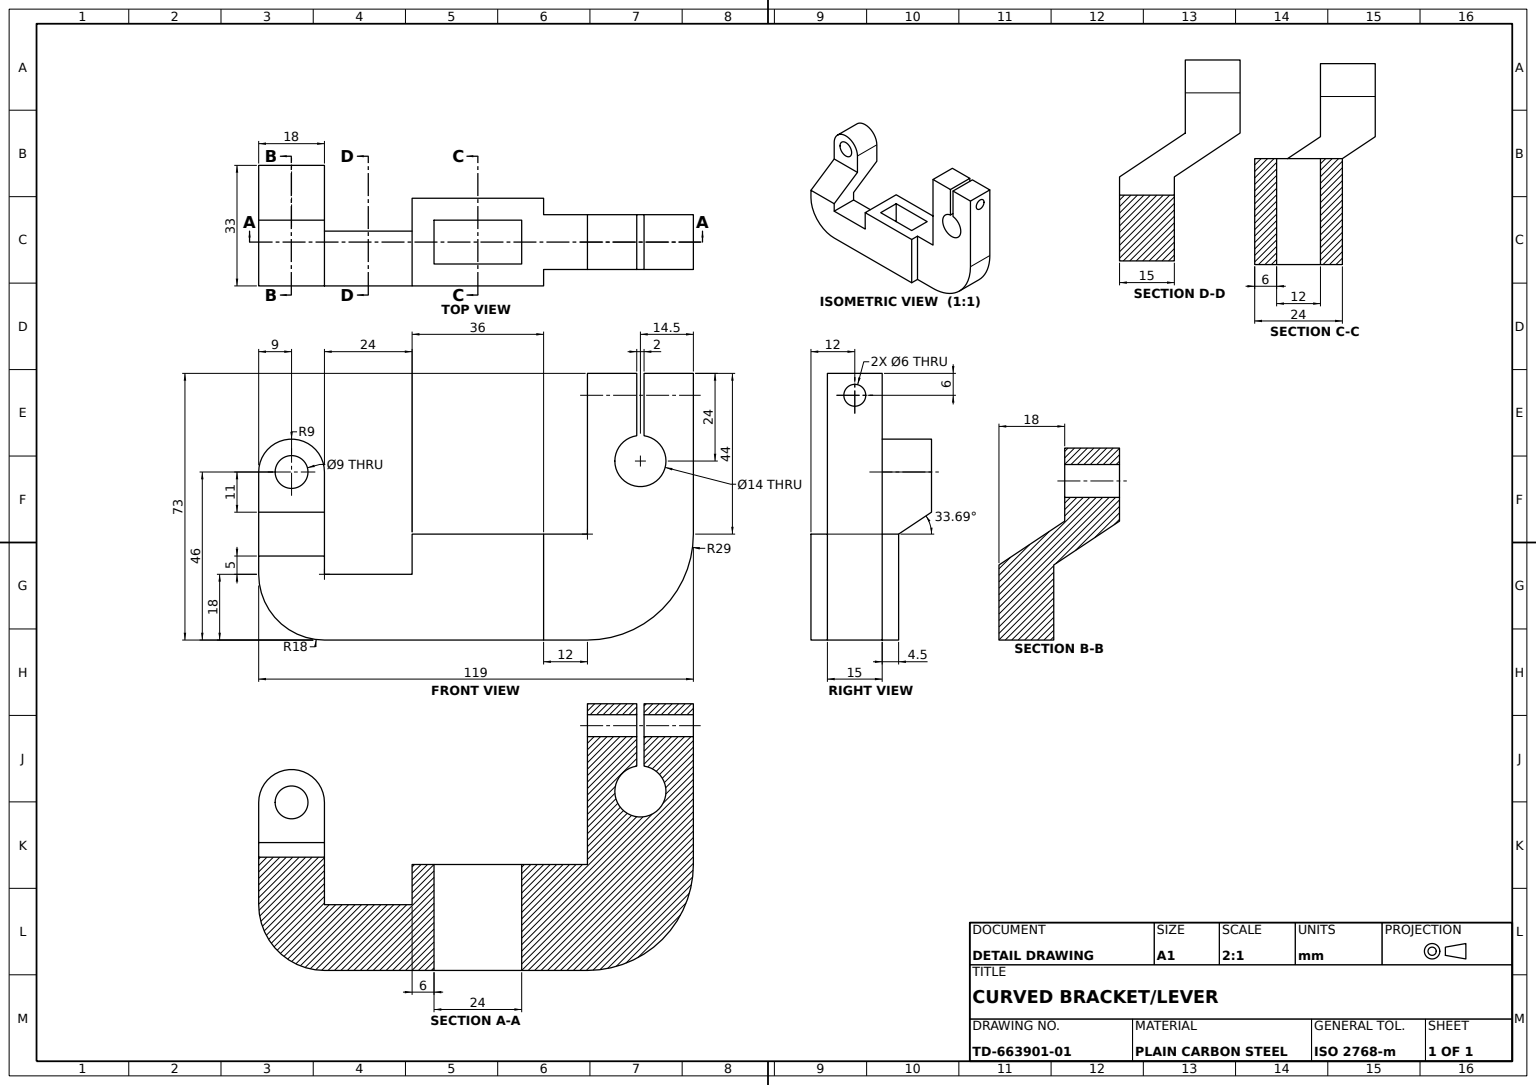
from build123d import *

# Parameters (mm, degrees)
BRACKET_BODY_DEPTH         = 12
BODY_RELIEF_CUT_DEPTH      = 75.57211275
BODY_RELIEF_CUT_DEPTH_BACK = 75.57211275
BODY_RELIEF_SKETCH_W       = 24
BODY_RELIEF_SKETCH_H       = 12
BODY_RELIEF_SKETCH_H_2     = 9
BODY_RELIEF_SKETCH_W_2     = 41
BODY_RELIEF_SKETCH_H_3     = 4.5
RECTANGULAR_WINDOW_DEPTH   = 86.343423883
CLAMP_HOLE_SKETCH_R        = 3
CLAMP_HOLE_6_DEPTH         = 94.542770966
ARM_BOSS_DEPTH             = 15
PIVOT_LUG_DEPTH            = 18
LUG_FILL_BOSS_DEPTH        = 15
PIVOT_BORE_SKETCH_R        = 4.5
PIVOT_BORE_9_DEPTH         = 24


with BuildPart() as part:
    # Bracket Profile Sketch → Bracket Body (new, symmetric)
    with BuildSketch(Plane.XY):
        with BuildLine():
            Line((30, 14.5), (30, 58.5))
            Line((30, 58.5), (59, 58.5))
            Line((59, 58.5), (59, 14.5))
            ThreePointArc((59, 14.5), (50.506096654, -6.006096654), (30, -14.5))
            Line((30, -14.5), (18, -14.5))
            Line((18, -14.5), (-18, -14.5))
            Line((-18, -14.5), (-42, -14.5))
            Line((-42, -14.5), (-42, 3.5))
            Line((-42, 3.5), (-18, 3.5))
            Line((-18, 3.5), (-18, 14.5))
            Line((-18, 14.5), (18, 14.5))
            Line((18, 14.5), (30, 14.5))
        make_face()
    extrude(amount=BRACKET_BODY_DEPTH, both=True)

    # Body Relief Sketch → Body Relief Cut (cut, two sides: drawn at the far end of the back side and taken through both)
    with BuildSketch(Plane(origin=(0, 14.5, 0), x_dir=(1, 0, 0), z_dir=(0, 1, 0)).offset(-BODY_RELIEF_CUT_DEPTH_BACK)):
        Rectangle(BODY_RELIEF_SKETCH_W, BODY_RELIEF_SKETCH_H)
        with Locations((-30, 7.5)):
            Rectangle(BODY_RELIEF_SKETCH_W, BODY_RELIEF_SKETCH_H_2)
        with Locations((38.5, -9.75)):
            Rectangle(BODY_RELIEF_SKETCH_W_2, BODY_RELIEF_SKETCH_H_3)
        with Locations((38.5, 9.75)):
            Rectangle(BODY_RELIEF_SKETCH_W_2, BODY_RELIEF_SKETCH_H_3)
    extrude(amount=BODY_RELIEF_CUT_DEPTH + BODY_RELIEF_CUT_DEPTH_BACK, mode=Mode.SUBTRACT)

    # Window Sketch → Rectangular Window (cut, through all)
    with BuildSketch(Plane.XY.offset(7.5)):
        with BuildLine():
            Line((43.5, 41.42820323), (43.5, 58.5))
            Line((43.5, 58.5), (45.5, 58.5))
            Line((45.5, 58.5), (45.5, 41.42820323))
            ThreePointArc((45.5, 41.42820323), (44.5, 27.5), (43.5, 41.42820323))
        make_face()
    extrude(amount=-RECTANGULAR_WINDOW_DEPTH, mode=Mode.SUBTRACT)

    # Clamp Hole Sketch → Clamp Hole Ø6 (cut, through all)
    with BuildSketch(Plane.ZY.offset(-30)):
        with Locations((0, 52.5)):
            Circle(CLAMP_HOLE_SKETCH_R)
    extrude(amount=-CLAMP_HOLE_6_DEPTH, mode=Mode.SUBTRACT)

    # Arm Sketch → Arm Boss (add)
    with BuildSketch(Plane.XY.offset(12)):
        with BuildLine():
            Line((-60, 3.5), (-60, 8.5))
            Line((-60, 8.5), (-42, 8.5))
            Line((-42, 8.5), (-42, 3.5))
            Line((-42, 3.5), (-42, -14.5))
            ThreePointArc((-42, -14.5), (-54.727922061, -9.227922061), (-60, 3.5))
        make_face()
    extrude(amount=-ARM_BOSS_DEPTH)

    # Pivot Lug Sketch → Pivot Lug (add)
    with BuildSketch(Plane.ZY.offset(60)):
        Polygon((-3, 8.5), (-21, 20.5), (-21, 31.5), (-6, 31.5), (-6, 20.5), (12, 8.5), align=None)
    extrude(amount=-PIVOT_LUG_DEPTH)

    # Lug Fill Sketch → Lug Fill Boss (add)
    with BuildSketch(Plane.XY.offset(-6)):
        with BuildLine():
            Line((-60, 31.5), (-42, 31.5))
            ThreePointArc((-42, 31.5), (-51, 40.5), (-60, 31.5))
        make_face()
    extrude(amount=-LUG_FILL_BOSS_DEPTH)

    # Pivot Bore Sketch → Pivot Bore Ø9 (cut)
    with BuildSketch(Plane.XY.offset(-6)):
        with Locations((-51, 31.5)):
            Circle(PIVOT_BORE_SKETCH_R)
    extrude(amount=-PIVOT_BORE_9_DEPTH, mode=Mode.SUBTRACT)


solid = part.part
